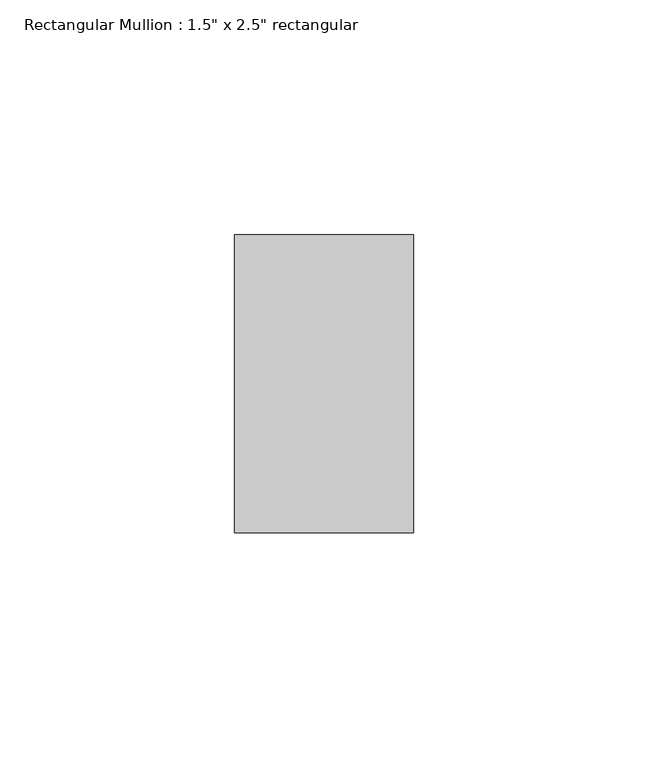
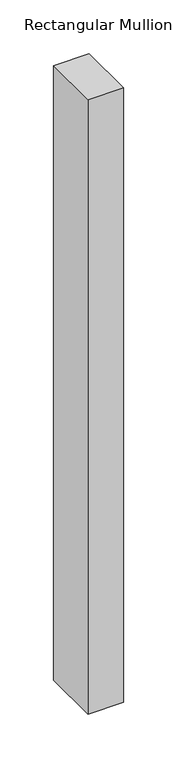
"""IFC4 building model written with IfcOpenShell, lengths in millimetres: member geometry."""

from ifc_helpers import new_model, si_unit, frame, origin, place, context, project, spatial, polyline, outline, extrude, source, transform, mapped, element, save


def member_85007bd8(model_context):
    return source(origin(), model_context, "Body", "SweptSolid", [
        extrude(outline(polyline([(19.05, 31.75), (19.05, -31.75), (-19.05, -31.75), (-19.05, 31.75), (19.05, 31.75)])), frame((0.0, 0.0, -696.6966705), z_axis=(0.0, 0.0, 1.0), x_axis=(1.0, 0.0, 0.0)), (0.0, 0.0, 1.0), 696.6966705),
    ])


if __name__ == "__main__":
    model = new_model("IFC4")
    model_context = context("Model", 3, world=origin())
    ifc_project = project(units=[si_unit("LENGTHUNIT", "METRE", prefix="MILLI")], contexts=[model_context])
    site = spatial("IfcSite", under=ifc_project)
    building = spatial("IfcBuilding", under=site)
    placement = place(None, origin())
    member_shape = member_85007bd8(model_context)
    element("IfcMember", 1, ObjectType="Rectangular Mullion : 1.5\" x 2.5\" rectangular", at=placement, inside=building, context=model_context, shape_type="MappedRepresentation", body=[
        mapped(member_shape, transform((0.0, 0.0, 0.0), x_axis=(1.0, 0.0, 0.0), y_axis=(0.0, 1.0, 0.0), z_axis=(0.0, 0.0, 1.0))),
    ])
    save(model, "model.ifc")

# Revit data of these elements
# Type "Rectangular Mullion : 1.5\" x 2.5\" rectangular"
#   built-in parameter 1007304 = 0.208333 (stored number, unit not read)
#   built-in parameter 1007301 = 0.0625 (stored number, unit not read)
#   built-in parameter 1007300 = 0.0625 (stored number, unit not read)
# Element 1 (IfcMember, "Rectangular Mullion : 1.5\" x 2.5\" rectangular")
#   Materials on its faces: "Damp-proofing"
# Materials
#   "Damp-proofing": class "Generic", colour RGB 127 127 127, transparency 0, Description = "Damp-proofing", Cost = 0
